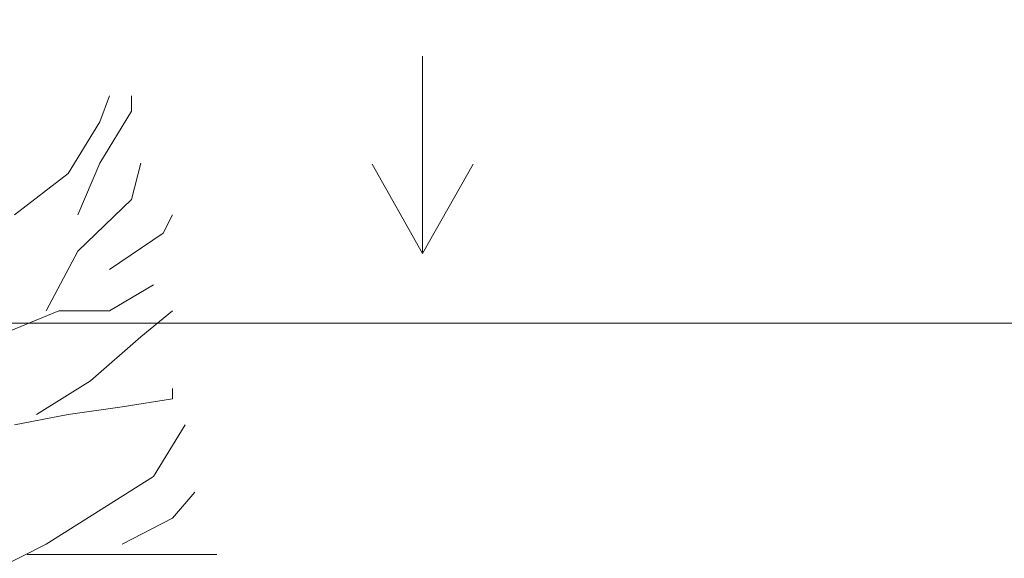
# Model space of a CAD drawing. Units: millimetres. Extents: x 595116 to 630915, y 909473 to 920225.
# Tile 27 of 134: x 629596 to 629613, y 919181 to 919190. Entities that reach past the tile are written whole.
import ezdxf

# ---------------------------------------------------------------- set-up
doc = ezdxf.new("R2010")
doc.units = ezdxf.units.MM
doc.layers.add('Dimension', color=3, linetype='Continuous', lineweight=18)
doc.layers.add('L-PLNT', color=85, linetype='Continuous', lineweight=13)
doc.styles.get("Standard").update_dxf_attribs({"font": 'arial.ttf'})
doc.dimstyles.new('ISO-25', dxfattribs={"dimtxt": 9, "dimasz": 6, "dimexe": 1.25, "dimexo": 0.625, "dimtad": 1, "dimlunit": 4, "dimtxsty": 'Standard', "dimcen": 2.5, "dimadec": 0, "dimazin": 0, "dimtfac": 1, "dimtmove": 0, "dimatfit": 3, "dimfxl": 1, "dimarcsym": 0})

# ---------------------------------------------------------------- blocks, each defined once
blk = doc.blocks.new('A$C143125F4')
for p, q in [((4.7101, 3.1717), (4.7265, 3.2165)), ((4.7648, 3.1897), (4.7648, 3.2165)), ((4.7101, 3.1001), (4.7648, 3.1897)), ((4.6554, 3.0821), (4.7101, 3.1717)), ((4.6718, 3.0105), (4.7101, 3.1001)), ((4.7648, 3.0373), (4.7812, 3.1001)), ((4.5624, 3.0105), (4.6554, 3.0821)), ((4.6718, 2.9477), (4.7648, 3.0373)), ((4.8195, 2.9791), (4.8359, 3.0105)), ((4.7265, 2.9164), (4.8195, 2.9791)), ((4.6171, 2.8447), (4.6718, 2.9477)), ((4.7265, 2.8447), (4.8031, 2.8895)), ((4.5296, 2.7999), (4.639, 2.8447)), ((4.639, 2.8447), (4.7265, 2.8447)), ((4.7812, 2.7999), (4.8359, 2.8447)), ((4.6937, 2.7238), (4.7812, 2.7999)), ((4.6007, 2.6655), (4.6937, 2.7238)), ((4.8359, 2.6924), (4.8359, 2.7103)), ((4.7484, 2.679), (4.8359, 2.6924)), ((4.6554, 2.6655), (4.7484, 2.679)), ((4.5624, 2.6476), (4.6554, 2.6655)), ((4.8031, 2.558), (4.8578, 2.6476)), ((4.6171, 2.4415), (4.8031, 2.558)), ((4.8359, 2.4863), (4.8742, 2.5311)), ((4.7484, 2.4415), (4.8359, 2.4863)), ((4.5296, 2.3967), (4.6171, 2.4415)), ((4.5843, 2.4236), (4.9125, 2.4236))]:
    blk.add_line(p, q)
blk = doc.blocks.new('LAWN-GRASS-TUFT')
blk.add_line((0.892, 3.485), (0.892, 0))
blk.add_lwpolyline([(0, 1.577), (0.892, 0), (1.785, 1.577)])
blk = doc.blocks.new('*D216')
at = {"layer": 'Defpoints', "color": 0, "transparency": 16777216}
for p in [(629743.541, 919411.928), (629505.041, 919411.828), (629743.541, 918832.378)]:
    blk.add_point(p, dxfattribs=at)
at = {"layer": 'Dimension', "color": 0, "lineweight": -2, "transparency": 16777216}
for p, q in [((629743.541, 919411.303), (629743.541, 918831.128)), ((629505.041, 919411.203), (629505.041, 918831.128)), ((629511.041, 918832.378), (629737.541, 918832.378))]:
    blk.add_line(p, q, dxfattribs=at)
at = {"layer": 'Dimension', "color": 0, "transparency": 16777216}
for points in [[(629511.041, 918833.378), (629511.041, 918831.378), (629505.041, 918832.378)], [(629737.541, 918833.378), (629737.541, 918831.378), (629743.541, 918832.378)]]:
    blk.add_solid(points, dxfattribs=at)
at = {"layer": 'Dimension', "color": 0, "transparency": 16777216, "insert": (629624.291, 918837.656), "char_height": 9, "attachment_point": 5}
blk.add_mtext('19\'-10 1/2"', dxfattribs=at)

msp = doc.modelspace()

# ---------------------------------------------------------------- linework, layer by layer
at = {"layer": 'L-PLNT'}
msp.add_line((629535.274, 919184.917), (629800.951, 919184.917), dxfattribs=at)

# ---------------------------------------------------------------- block references
at = {"layer": 'L-PLNT', "xscale": 10.20167662382051, "yscale": 10.20167662382051, "zscale": 10.20167662382051}
msp.add_blockref('A$C143125F4', (629549.214, 919156.111), dxfattribs=at)
at = {"layer": 'L-PLNT'}
msp.add_blockref('LAWN-GRASS-TUFT', (629602.065, 919186.14), dxfattribs=at)

# ---------------------------------------------------------------- dimensions: what is measured, and where the dimension line sits
at = {"layer": 'Dimension'}
dim = msp.add_linear_dim(base=(629743.541, 918832.378), p1=(629505.041, 919411.828), p2=(629743.541, 919411.928), dimstyle='ISO-25', override={"dimdec": 1, "dimlfac": 1, "dimrnd": 0, "dimzin": 1, "dimdsep": 46, "dimlunit": 4, "dimfrac": 2}, dxfattribs=at)
dim.commit()
dim.dimension.update_dxf_attribs({"geometry": '*D216', "text_midpoint": (629624.291, 918837.656)})

doc.saveas('drawing.dxf')
